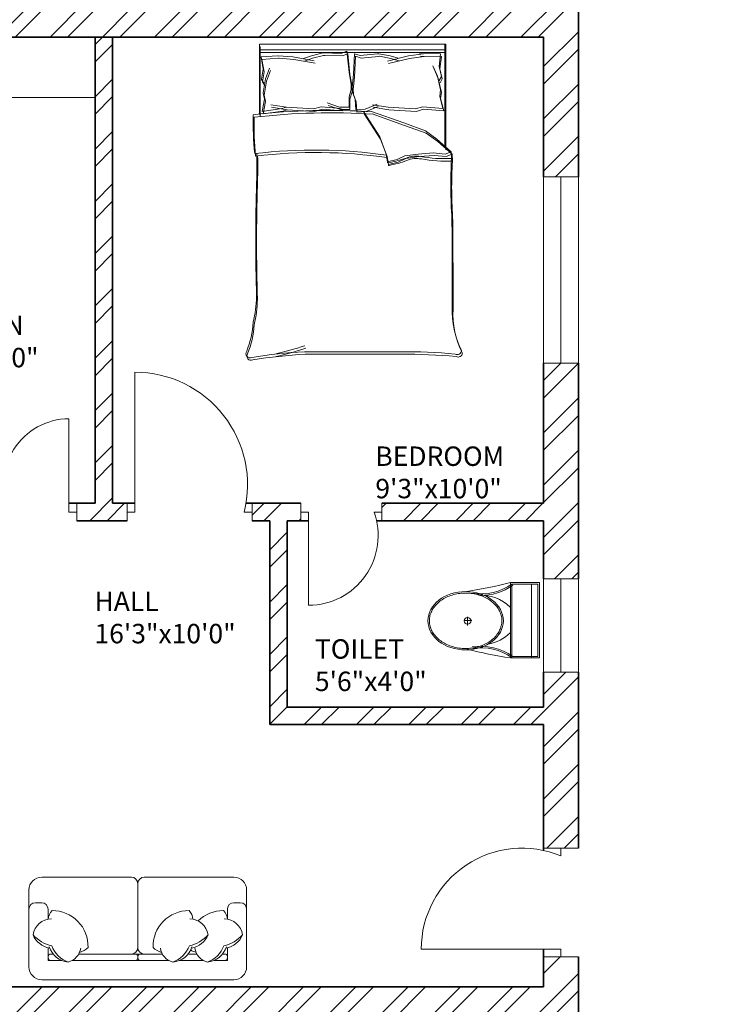
# Model space of a CAD drawing. Units: inches. Extents: x 2552 to 3217, y 1417 to 2737.
# Tile 8 of 25: x 2705 to 2885, y 1885 to 2138. Entities that reach past the tile are written whole.
import ezdxf

# ---------------------------------------------------------------- set-up
doc = ezdxf.new("R2010")
doc.units = ezdxf.units.IN
for name, color, linetype, lineweight in [('A-ANNO-DIMS', 2, 'Continuous', 18), ('A-AREA-IDEN', 7, 'Continuous', 18), ('A-DOOR', 21, 'Continuous', 18), ('A-FLOR-CASE', 9, 'Continuous', 18), ('A-FLOR-FIXT', 8, 'Continuous', 18), ('A-FURN', 8, 'Continuous', 13), ('A-GLAZ', 161, 'Continuous', 18), ('A-WALL', 7, 'Continuous', 35), ('A-WALL-PATT', 217, 'Continuous', 13)]:
    doc.layers.add(name, color=color, linetype=linetype, lineweight=lineweight)
doc.styles.get("Standard").update_dxf_attribs({"font": 'arial.ttf'})
doc.dimstyles.get("Standard").update_dxf_attribs({"dimtxt": 0.18, "dimasz": 0.18, "dimexe": 0.18, "dimexo": 0.0625, "dimgap": 0.09, "dimtad": 0, "dimtih": 1, "dimtoh": 1, "dimdec": 4, "dimzin": 0, "dimdsep": 46, "dimtxsty": 'Standard', "dimcen": 0.09, "dimadec": 0, "dimazin": 0, "dimtfac": 1, "dimtdec": 4, "dimtofl": 0, "dimtmove": 0, "dimatfit": 3, "dimfxl": 1, "dimtolj": 1, "dimtzin": 0, "dimarcsym": 0})

# ---------------------------------------------------------------- blocks, each defined once
blk = doc.blocks.new('A$C31115884')
for p, q in [((283.1, 497.7), (223.4, 497.7)), ((257.5, 466.4), (257.5, 523.2)), ((0, 200), (0, 0)), ((520, 200), (0, 200)), ((10, 190), (10, 10)), ((510, 190), (10, 190)), ((510, 10), (510, 190)), ((520, 0), (520, 200)), ((510, 54.5), (0, 54.5)), ((10, 10), (510, 10)), ((0, 0), (520, 0))]:
    blk.add_line(p, q)
blk.add_circle((255.6, 496.4), 23.6)
for centre, radius, start, end in [((2777.7, -204.6), 2807, 165.4549, 171.71327), ((3237, 905), 2807, 188.28673, 194.5451), ((-294.5, 403.3), 364.7, 324.20913, 9.34987), ((-294.5, 403.3), 374.7, 324.20913, 9.34987), ((139.5, 406.2), 293.5, 315.84364, 2.65635), ((805.8, 403.3), 374.7, 179.20365, 215.79087), ((805.8, 403.3), 364.7, 170.65013, 215.79087), ((383.6, 406.2), 293.5, 190.27735, 224.15636)]:
    blk.add_arc(centre, radius, start, end)
blk.add_ellipse((256.2, 509.9), major_axis=(0, -260.7), ratio=0.772727)
blk.add_open_spline([(256.2, 259.2), (263.1, 259.2), (270, 259.7), (287.8, 262.3), (298.7, 265.1), (319.9, 273.1), (330.2, 278.4), (350.1, 291.1), (359.7, 298.7), (377.7, 315.9), (386.2, 325.5), (401.7, 346.6), (408.8, 358.1), (421.3, 382.5), (426.8, 395.5), (435.9, 422.4), (439.5, 436.4), (444.8, 465.1), (446.5, 479.7), (447.9, 509.2), (447.6, 524), (445, 553.3), (442.7, 567.8), (436.3, 596), (432.1, 609.7), (421.9, 636), (416, 648.6), (402.5, 672.1), (395, 683), (378.6, 703), (369.8, 712.1), (351.1, 728), (341.3, 734.8), (320.9, 746.2), (310.4, 750.7), (288.9, 757.3), (278, 759.4), (256, 761), (245, 760.6), (223.1, 757.2), (212.3, 754.3), (191.1, 746.1), (180.8, 740.7), (160.9, 727.8), (151.4, 720.1), (133.5, 702.7), (125.1, 693), (109.6, 671.7), (102.6, 660.2), (90.2, 635.7), (84.9, 622.7), (76, 595.6), (72.4, 581.6), (67.2, 552.9), (65.6, 538.2), (64.4, 508.8), (64.8, 494), (67.5, 464.7), (69.9, 450.2), (76.6, 422), (80.8, 408.3), (91.1, 382.2), (97.2, 369.7), (110.8, 346.3), (118.4, 335.4), (134.8, 315.6), (143.7, 306.7), (162.4, 290.9), (172.3, 284.2), (192.8, 273), (203.3, 268.6), (224.8, 262.2), (235.8, 260.2), (249.9, 259.3), (253, 259.2), (256.2, 259.2)], degree=3, knots=[0, 0, 0, 0, 0.110105, 0.110105, 0.285049, 0.285049, 0.459994, 0.459994, 0.634938, 0.634938, 0.809882, 0.809882, 0.984827, 0.984827, 1.159771, 1.159771, 1.334715, 1.334715, 1.50966, 1.50966, 1.684604, 1.684604, 1.859549, 1.859549, 2.034493, 2.034493, 2.209437, 2.209437, 2.384382, 2.384382, 2.559326, 2.559326, 2.73427, 2.73427, 2.909215, 2.909215, 3.084159, 3.084159, 3.259103, 3.259103, 3.434048, 3.434048, 3.608992, 3.608992, 3.783936, 3.783936, 3.958881, 3.958881, 4.133825, 4.133825, 4.30877, 4.30877, 4.483714, 4.483714, 4.658658, 4.658658, 4.833603, 4.833603, 5.008547, 5.008547, 5.183491, 5.183491, 5.358436, 5.358436, 5.53338, 5.53338, 5.708324, 5.708324, 5.883269, 5.883269, 6.058213, 6.058213, 6.233158, 6.233158, 6.283185, 6.283185, 6.283185, 6.283185])
blk = doc.blocks.new('BED-DOUBLE')
for p, q in [((3.47, 63.33), (3.47, 81.44)), ((3.47, 81.44), (51.49, 81.44)), ((3.48, 63.33), (3.48, 81.44)), ((51.27, 81.44), (51.27, 54.83)), ((51.27, 81.44), (51.27, 54.83)), ((51.49, 81.44), (51.49, 80.8)), ((3.47, 79.91), (51.27, 79.91)), ((3.48, 79.91), (51.27, 79.91)), ((3.7, 62.69), (3.7, 80.8)), ((3.7, 62.69), (3.7, 80.8)), ((3.7, 79.27), (51.49, 79.27)), ((3.7, 79.27), (51.49, 79.27)), ((16.88, 78.42), (19.77, 79.14)), ((16.88, 78.42), (19.77, 79.14)), ((19.77, 79.14), (20.09, 79.14)), ((19.77, 79.14), (20.09, 79.14)), ((20.09, 79.14), (24.54, 78.99)), ((20.09, 79.14), (24.54, 78.99)), ((24.54, 78.99), (25.98, 79.57)), ((24.54, 78.99), (25.98, 79.57)), ((24.77, 78.36), (26.21, 78.93)), ((24.77, 78.36), (26.21, 78.93)), ((25.98, 79.57), (26.56, 74.22)), ((25.98, 79.57), (26.56, 74.22)), ((26.21, 78.93), (26.79, 73.58)), ((26.21, 78.93), (26.79, 73.58)), ((27.98, 78.95), (27.73, 73.58)), ((27.98, 78.95), (27.73, 73.58)), ((29.46, 78.46), (27.98, 78.95)), ((29.46, 78.46), (27.98, 78.95)), ((33.88, 78.89), (29.46, 78.46)), ((33.88, 78.89), (29.46, 78.46)), ((34.2, 78.91), (33.88, 78.89)), ((34.2, 78.91), (33.88, 78.89)), ((37.14, 78.36), (34.2, 78.91)), ((37.14, 78.36), (34.2, 78.91)), ((45.71, 78.9), (41.91, 78.37)), ((45.71, 78.9), (41.91, 78.37)), ((50.11, 78.89), (44.71, 78.98)), ((44.71, 78.98), (45.71, 78.9)), ((50.11, 78.89), (44.71, 78.98)), ((44.71, 78.98), (45.71, 78.9)), ((50.11, 78.89), (49.73, 75.68)), ((50.11, 78.89), (49.73, 75.68)), ((51.49, 80.8), (51.49, 54.19)), ((51.49, 80.8), (51.49, 54.19)), ((3.89, 78.13), (4.47, 74.95)), ((3.89, 78.13), (4.47, 74.95)), ((3.9, 78.11), (8.18, 78.43)), ((3.9, 78.11), (8.18, 78.43)), ((4.12, 77.49), (4.7, 74.31)), ((4.12, 77.49), (4.7, 74.31)), ((4.13, 77.47), (8.41, 77.8)), ((4.13, 77.47), (8.41, 77.8)), ((8.18, 78.43), (8.28, 78.42)), ((8.18, 78.43), (8.28, 78.42)), ((8.28, 78.42), (12.11, 78.13)), ((8.28, 78.42), (12.11, 78.13)), ((8.41, 77.8), (8.51, 77.78)), ((8.41, 77.8), (8.51, 77.78)), ((8.51, 77.78), (12.34, 77.49)), ((8.51, 77.78), (12.34, 77.49)), ((12.11, 78.13), (17.6, 77.12)), ((12.11, 78.13), (17.6, 77.12)), ((12.34, 77.49), (17.83, 76.48)), ((12.34, 77.49), (17.83, 76.48)), ((14.85, 77.69), (16.88, 78.42)), ((14.85, 77.69), (16.88, 78.42)), ((15.08, 77.05), (17.11, 77.78)), ((15.08, 77.05), (17.11, 77.78)), ((17.11, 77.78), (20, 78.5)), ((17.11, 77.78), (20, 78.5)), ((20, 78.5), (20.32, 78.5)), ((20, 78.5), (20.32, 78.5)), ((20.32, 78.5), (24.77, 78.36)), ((20.32, 78.5), (24.77, 78.36)), ((28.21, 78.31), (27.96, 72.94)), ((28.21, 78.31), (27.96, 72.94)), ((29.68, 77.83), (28.21, 78.31)), ((29.68, 77.83), (28.21, 78.31)), ((34.11, 78.25), (29.68, 77.83)), ((34.11, 78.25), (29.68, 77.83)), ((34.43, 78.27), (34.11, 78.25)), ((34.43, 78.27), (34.11, 78.25)), ((37.36, 77.73), (34.43, 78.27)), ((37.36, 77.73), (34.43, 78.27)), ((41.91, 78.37), (36.49, 77.02)), ((41.91, 78.37), (36.5, 77.02)), ((42.14, 77.73), (36.72, 76.38)), ((42.14, 77.73), (36.72, 76.38)), ((39.2, 77.77), (37.14, 78.36)), ((39.2, 77.77), (37.14, 78.36)), ((39.43, 77.13), (37.36, 77.73)), ((39.43, 77.13), (37.36, 77.73)), ((45.94, 78.26), (42.14, 77.73)), ((45.94, 78.26), (42.14, 77.73)), ((50.34, 78.25), (44.94, 78.34)), ((44.94, 78.34), (45.94, 78.26)), ((50.34, 78.25), (44.94, 78.34)), ((44.94, 78.34), (45.94, 78.26)), ((50.34, 78.25), (49.96, 75.04)), ((50.34, 78.25), (49.96, 75.04)), ((4.47, 74.95), (4.04, 72.34)), ((4.47, 74.95), (4.04, 72.34)), ((4.7, 74.31), (4.27, 71.7)), ((4.7, 74.31), (4.27, 71.7)), ((5.05, 72.49), (6.06, 75.24)), ((5.05, 72.49), (6.06, 75.24)), ((5.28, 71.85), (6.29, 74.6)), ((5.28, 71.85), (6.29, 74.6)), ((26.56, 74.22), (27.14, 71.04)), ((26.56, 74.22), (27.14, 71.04)), ((26.79, 73.58), (27.37, 70.4)), ((26.79, 73.58), (27.37, 70.4)), ((27.73, 73.58), (27.35, 70.37)), ((27.73, 73.58), (27.35, 70.37)), ((49.31, 73.19), (48.13, 75.86)), ((49.31, 73.19), (48.13, 75.86)), ((49.54, 72.55), (48.36, 75.23)), ((49.54, 72.55), (48.36, 75.23)), ((49.73, 75.68), (50.33, 73.1)), ((49.73, 75.68), (50.33, 73.1)), ((49.96, 75.04), (50.56, 72.47)), ((49.96, 75.04), (50.56, 72.47)), ((4.04, 72.34), (4.62, 71.33)), ((4.04, 72.34), (4.62, 71.33)), ((4.27, 71.7), (4.85, 70.69)), ((4.27, 71.7), (4.85, 70.69)), ((4.47, 68.87), (5.05, 72.49)), ((4.47, 68.87), (5.05, 72.49)), ((4.7, 68.23), (5.28, 71.85)), ((4.7, 68.23), (5.28, 71.85)), ((27.14, 71.04), (27.14, 69.74)), ((27.14, 71.04), (27.14, 69.74)), ((27.96, 72.94), (27.58, 69.73)), ((27.96, 72.94), (27.58, 69.73)), ((50.11, 69.61), (49.31, 73.19)), ((50.11, 69.61), (49.31, 73.19)), ((50.34, 68.98), (49.54, 72.55)), ((50.34, 68.98), (49.54, 72.55)), ((50.33, 73.1), (49.81, 72.06)), ((50.33, 73.1), (49.81, 72.06)), ((50.56, 72.47), (50.04, 71.42)), ((50.56, 72.47), (50.04, 71.42)), ((4.76, 67.28), (4.47, 68.87)), ((4.76, 67.28), (4.47, 68.87)), ((27.14, 69.74), (26.56, 67.86)), ((27.14, 69.74), (26.56, 67.86)), ((27.37, 69.1), (26.79, 67.22)), ((27.37, 69.1), (26.79, 67.22)), ((27.35, 70.37), (27.44, 69.07)), ((27.35, 70.37), (27.44, 69.07)), ((27.37, 70.4), (27.37, 69.1)), ((27.37, 70.4), (27.37, 69.1)), ((27.44, 69.07), (28.13, 67.23)), ((27.44, 69.07), (28.13, 67.23)), ((27.58, 69.73), (27.66, 68.43)), ((27.58, 69.73), (27.66, 68.43)), ((49.92, 68.01), (50.11, 69.61)), ((49.92, 68.01), (50.11, 69.61)), ((50.15, 67.37), (50.34, 68.98)), ((50.15, 67.37), (50.34, 68.98)), ((4.18, 64.1), (4.76, 67.28)), ((4.18, 64.1), (4.76, 67.28)), ((4.41, 63.46), (4.99, 66.64)), ((4.41, 63.46), (4.99, 66.64)), ((4.99, 66.64), (4.7, 68.23)), ((4.99, 66.64), (4.7, 68.23)), ((24.1, 65.18), (20.96, 66.27)), ((24.1, 65.18), (20.96, 66.27)), ((26.56, 67.86), (26.56, 65.18)), ((26.56, 67.86), (26.56, 65.18)), ((26.79, 67.22), (26.79, 64.54)), ((26.79, 67.22), (26.79, 64.54)), ((27.66, 68.43), (28.36, 66.59)), ((27.66, 68.43), (28.36, 66.59)), ((28.13, 67.23), (28.3, 64.55)), ((28.13, 67.23), (28.3, 64.55)), ((28.36, 66.59), (28.53, 63.91)), ((28.36, 66.59), (28.53, 63.91)), ((30.75, 64.7), (33.82, 65.99)), ((30.75, 64.7), (33.82, 65.99)), ((50.7, 64.87), (49.92, 68.01)), ((50.7, 64.87), (49.92, 68.01)), ((50.93, 64.23), (50.15, 67.37)), ((50.93, 64.23), (50.15, 67.37)), ((9.28, 64.83), (4.18, 64.1)), ((9.28, 64.83), (4.18, 64.1)), ((9.51, 64.19), (4.41, 63.46)), ((9.51, 64.19), (4.41, 63.46)), ((6.38, 65.81), (10.41, 65.15)), ((6.38, 65.81), (10.41, 65.15)), ((6.61, 65.18), (10.64, 64.51)), ((6.61, 65.18), (10.64, 64.51)), ((10.41, 65.15), (9.28, 64.83)), ((10.41, 65.15), (9.28, 64.83)), ((10.64, 64.51), (9.51, 64.19)), ((10.64, 64.51), (9.51, 64.19)), ((10.41, 65.15), (17.42, 64.72)), ((10.41, 65.15), (17.42, 64.72)), ((10.64, 64.51), (17.65, 64.08)), ((10.64, 64.51), (17.65, 64.08)), ((17.42, 64.72), (19.38, 65.27)), ((17.42, 64.72), (19.38, 65.27)), ((17.65, 64.08), (19.61, 64.63)), ((17.65, 64.08), (19.61, 64.63)), ((19.38, 65.27), (24.52, 64.87)), ((19.38, 65.27), (24.52, 64.87)), ((19.61, 64.63), (24.74, 64.23)), ((19.61, 64.63), (24.74, 64.23)), ((24.33, 64.54), (21.19, 65.63)), ((24.33, 64.54), (21.19, 65.63)), ((26.56, 65.18), (24.1, 65.18)), ((26.56, 65.18), (24.1, 65.18)), ((26.79, 64.54), (24.33, 64.54)), ((26.79, 64.54), (24.33, 64.54)), ((28.3, 64.55), (30.75, 64.7)), ((28.3, 64.55), (30.75, 64.7)), ((28.53, 63.91), (30.98, 64.06)), ((28.53, 63.91), (30.98, 64.06)), ((30.26, 64.06), (34.45, 57.57)), ((30.26, 64.06), (34.45, 57.57)), ((30.49, 63.42), (34.68, 56.93)), ((30.49, 63.42), (34.68, 56.93)), ((30.98, 64.06), (34.05, 65.35)), ((30.98, 64.06), (34.05, 65.35)), ((40.64, 61.13), (32.31, 64.06)), ((40.64, 61.13), (32.31, 64.06)), ((40.87, 60.49), (32.53, 63.42)), ((40.87, 60.49), (32.53, 63.42)), ((32.56, 65.81), (36.6, 65.15)), ((32.56, 65.81), (36.6, 65.15)), ((32.79, 65.18), (36.82, 64.51)), ((32.79, 65.18), (36.82, 64.51)), ((36.6, 65.15), (43.61, 64.72)), ((36.6, 65.15), (43.61, 64.72)), ((36.82, 64.51), (43.83, 64.08)), ((36.82, 64.51), (43.83, 64.08)), ((43.61, 64.72), (45.57, 65.27)), ((43.61, 64.72), (45.57, 65.27)), ((43.83, 64.08), (45.79, 64.63)), ((43.83, 64.08), (45.79, 64.63)), ((45.57, 65.27), (50.7, 64.87)), ((45.57, 65.27), (50.7, 64.87)), ((45.79, 64.63), (50.93, 64.23)), ((45.79, 64.63), (50.93, 64.23)), ((46.22, 59.11), (40.64, 61.13)), ((46.22, 59.11), (40.64, 61.13)), ((46.45, 58.48), (40.87, 60.49)), ((46.45, 58.48), (40.87, 60.49)), ((49.16, 56.95), (46.22, 59.11)), ((49.16, 56.95), (46.22, 59.11)), ((49.39, 56.31), (46.45, 58.48)), ((49.39, 56.31), (46.45, 58.48)), ((34.45, 57.57), (36.15, 53.08)), ((34.45, 57.57), (36.15, 53.08)), ((34.68, 56.93), (36.38, 52.44)), ((34.68, 56.93), (36.38, 52.44)), ((52.87, 53.7), (49.16, 56.95)), ((52.87, 53.7), (49.16, 56.95)), ((53.1, 53.06), (49.39, 56.31)), ((53.1, 53.06), (49.39, 56.31)), ((44.36, 53.08), (48.23, 53.39)), ((44.36, 53.08), (48.23, 53.39)), ((48.23, 53.39), (51.33, 53.08)), ((48.23, 53.39), (51.33, 53.08)), ((51.33, 53.08), (52.87, 53.7)), ((51.33, 53.08), (52.87, 53.7)), ((52.95, 51.95), (52.87, 53.7, 3.87)), ((52.95, 51.95), (52.87, 53.7, 3.87)), ((36.15, 53.08), (36.46, 51.07)), ((36.15, 53.08), (36.46, 51.07)), ((36.38, 52.44), (36.69, 50.43)), ((36.38, 52.44), (36.69, 50.43)), ((36.46, 51.07), (38.94, 51.69)), ((36.46, 51.07), (38.94, 51.69)), ((36.69, 50.43), (39.17, 51.05)), ((36.69, 50.43), (39.17, 51.05)), ((38.94, 51.69), (40.95, 52.61)), ((38.94, 51.69), (40.95, 52.61)), ((39.17, 51.05), (41.18, 51.97)), ((39.17, 51.05), (41.18, 51.97)), ((40.95, 52.61), (44.36, 53.08)), ((40.95, 52.61), (44.36, 53.08)), ((41.18, 51.97), (44.59, 52.44)), ((41.18, 51.97), (44.59, 52.44)), ((44.59, 52.44), (48.46, 52.75)), ((44.59, 52.44), (48.46, 52.75)), ((48.46, 52.75), (51.56, 52.44)), ((48.46, 52.75), (51.56, 52.44)), ((51.56, 52.44), (53.1, 53.06)), ((51.56, 52.44), (53.1, 53.06)), ((53.18, 51.31), (53.1, 53.06, 3.87)), ((53.18, 51.31), (53.1, 53.06, 3.87)), ((15.06, 2.2), (39.68, 2.2)), ((15.06, 2.2), (39.68, 2.2)), ((15.29, 1.56), (39.91, 1.56)), ((15.29, 1.56), (39.91, 1.56))]:
    blk.add_line(p, q)
for centre, radius, start, end in [((21.36, -100.61), 164.97, 86.0865, 96.7821), ((21.36, -100.61), 164.97, 86.0865, 96.7821), ((21.59, -101.25), 164.97, 86.0865, 96.7821), ((21.59, -101.25), 164.97, 86.0865, 96.7821), ((85.16, 61.35), 83.31, 178.7218, 185.604), ((85.16, 61.35), 83.31, 178.7218, 185.604), ((85.39, 60.71), 83.31, 178.7218, 185.604), ((85.39, 60.71), 83.31, 178.7218, 185.604), ((17.76, -74.87), 129.02, 81.7845, 96.9006), ((17.76, -74.87), 129.02, 81.7845, 96.9006), ((17.98, -75.51), 129.02, 81.7845, 96.9006), ((17.98, -75.51), 129.02, 81.7845, 96.9006), ((-167.31, 50.27), 170.11, 358.4762, 1.0082), ((-167.31, 50.27), 170.11, 358.4762, 1.0082), ((-167.08, 49.63), 170.11, 358.4762, 1.0082), ((-167.08, 49.63), 170.11, 358.4762, 1.0082), ((36.64, 51), 0.185, 160.2464, 271.1377), ((36.64, 51), 0.185, 160.2464, 271.1377), ((31.15, 79.96), 29.65, 280.6617, 289.8806), ((31.15, 79.96), 29.65, 280.6617, 289.8806), ((31.38, 79.32), 29.65, 280.6617, 289.8806), ((31.38, 79.32), 29.65, 280.6617, 289.8806), ((43.74, 46.38), 6.22, 78.6608, 113.7384), ((43.74, 46.38), 6.22, 78.6608, 113.7384), ((43.97, 45.74), 6.22, 78.6608, 113.7384), ((43.97, 45.74), 6.22, 78.6608, 113.7384), ((51.33, 88.1), 36.18, 259.8763, 272.5657), ((51.33, 88.1), 36.18, 259.8763, 272.5657), ((51.56, 87.46), 36.18, 259.8763, 272.5657), ((51.56, 87.46), 36.18, 259.8763, 272.5657), ((182.27, 45.13), 129.5, 176.9791, 183.8365), ((182.27, 45.13), 129.5, 176.9791, 183.8365), ((182.49, 44.49), 129.5, 176.9791, 183.8365), ((182.49, 44.49), 129.5, 176.9791, 183.8365), ((36.86, 50.36), 0.185, 160.2464, 271.1377), ((36.86, 50.36), 0.185, 160.2464, 271.1377), ((484.82, 30.83), 482.31, 178.2277, 181.7185), ((484.82, 30.83), 482.31, 178.2277, 181.7185), ((485.05, 30.19), 482.31, 178.2277, 181.7185), ((485.05, 30.19), 482.31, 178.2277, 181.7185), ((-4508.74, 13.62), 4561.86, 0.00217, 0.28689), ((-4508.74, 13.62), 4561.86, 0.00217, 0.28689), ((-4508.51, 12.98), 4561.86, 0.00217, 0.28689), ((-4508.52, 12.98), 4561.86, 0.00217, 0.28689), ((-26.9, 16.93), 29.63, 346.0648, 358.9113), ((-26.9, 16.93), 29.63, 346.0648, 358.9113), ((-26.67, 16.29), 29.63, 346.0648, 358.9113), ((-26.67, 16.29), 29.63, 346.0648, 358.9113), ((76.16, 12.78), 23.07, 177.4714, 206.4681), ((76.16, 12.78), 23.07, 177.4714, 206.4681), ((76.39, 12.14), 23.07, 177.4714, 206.4681), ((76.39, 12.14), 23.07, 177.4714, 206.4681), ((-21.66, 11.17), 23.56, 337.9751, 356.652), ((-21.66, 11.17), 23.56, 337.9751, 356.652), ((-21.43, 10.53), 23.56, 337.9751, 356.652), ((-21.43, 10.53), 23.56, 337.9751, 356.652), ((-17.22, 105.16), 106.46, 283.3832, 287.7053), ((-17.22, 105.16), 106.46, 283.3832, 287.7053), ((-16.99, 104.52), 106.46, 283.3832, 287.7053), ((-16.99, 104.52), 106.46, 283.3832, 287.7053), ((1.09, 1.73), 1.09, 146.1736, 293.4781), ((1.09, 1.73), 1.09, 146.1736, 293.4781), ((1.32, 1.09), 1.09, 146.1736, 293.4781), ((1.32, 1.09), 1.09, 146.1736, 293.4781), ((21.43, -119.39), 121.76, 92.9958, 99.4091), ((21.43, -119.39), 121.76, 92.9958, 99.4091), ((21.66, -120.03), 121.76, 92.9958, 99.4091), ((21.65, -120.03), 121.76, 92.9958, 99.4091), ((41.15, -130.83), 133.04, 84.4998, 90.6351), ((41.15, -130.83), 133.04, 84.4998, 90.6351), ((41.38, -131.47), 133.04, 84.4998, 90.6351), ((41.38, -131.47), 133.04, 84.4998, 90.6351), ((54.41, 2.57), 1.1, 242.6588, 356.02), ((54.41, 2.57), 1.1, 242.6588, 356.02), ((54.64, 1.93), 1.1, 242.6588, 356.02), ((54.64, 1.93), 1.1, 242.6588, 356.02)]:
    blk.add_arc(centre, radius, start, end)
blk = doc.blocks.new('WIN-48')
for p, q in [((4.5, 48), (0, 48)), ((0, 48), (9, 48)), ((0, 48), (0, 0)), ((4.5, 0), (4.5, 48)), ((9, 48), (9, 0)), ((0, 0), (9, 0)), ((9, 0), (4.5, 0))]:
    blk.add_line(p, q)
blk = doc.blocks.new('WIN-24')
for p, q in [((0, 24), (9, 24)), ((0, 24), (0, 0)), ((9, 24), (4.5, 24)), ((4.5, 24), (4.5, 0)), ((9, 24), (9, 0)), ((4.5, 0), (0, 0)), ((0, 0), (9, 0))]:
    blk.add_line(p, q)
blk = doc.blocks.new('*D64')
at = {"layer": 'A-ANNO-DIMS', "color": 0, "lineweight": -2, "transparency": 16777216}
for p, q in [((2646.35, 1551.58), (2646.35, 2709.49)), ((2646.53, 2709.31), (2802.77, 2709.31)), ((2959.93, 2709.31), (2803.69, 2709.31)), ((2960.11, 1551.58), (2960.11, 2709.49))]:
    blk.add_line(p, q, dxfattribs=at)
at = {"layer": 'A-ANNO-DIMS', "color": 0, "transparency": 16777216}
for points in [[(2646.53, 2709.34), (2646.53, 2709.28), (2646.35, 2709.31)], [(2959.93, 2709.34), (2959.93, 2709.28), (2960.11, 2709.31)]]:
    blk.add_solid(points, dxfattribs=at)
at = {"layer": 'Defpoints', "color": 0, "transparency": 16777216}
for p in [(2960.11, 2709.31), (2646.35, 1551.51), (2960.11, 1551.51)]:
    blk.add_point(p, dxfattribs=at)
at = {"layer": 'A-ANNO-DIMS', "color": 0, "transparency": 16777216, "insert": (2803.23, 2709.31), "char_height": 0.18, "attachment_point": 5}
blk.add_mtext('\\A1;313.76', dxfattribs=at)

msp = doc.modelspace()

# ---------------------------------------------------------------- hatches: boundary and pattern name
at = {"layer": 'A-WALL-PATT'}
h = msp.add_hatch(dxfattribs=at)
h.set_pattern_fill('ANSI32', color=256)
h.paths.add_polyline_path([(2756.676, 2649.5125), (2637.3535, 2649.5125), (2637.3535, 2617.9626), (2641.8535, 2617.9626), (2646.3535, 2617.9626), (2646.3535, 2640.5125), (2724.3535, 2640.5125), (2724.3535, 2520.5125), (2720.299, 2520.5125), (2720.299, 2516.0125), (2733.4075, 2516.0125), (2733.4075, 2518.2213), (2733.4075, 2520.5125), (2728.8535, 2520.5125), (2728.8535, 2640.5125), (2756.676, 2640.5125)])
h.paths.add_polyline_path([(2848.8535, 2649.5125), (2804.676, 2649.5125), (2804.676, 2640.5125), (2839.8535, 2640.5125), (2839.8535, 2598.3517), (2848.8535, 2598.3517)])
h.paths.add_polyline_path([(2646.3535, 2516.0125), (2697.9593, 2516.0125), (2697.9593, 2518.2625), (2697.9593, 2520.5125), (2646.3535, 2520.5125), (2646.3535, 2581.9626), (2637.3535, 2581.9626), (2637.3535, 2364.3298), (2646.3535, 2364.3298), (2646.3535, 2387.0125), (2724.3535, 2387.0125), (2724.3535, 2267.0125), (2721.0443, 2267.0125), (2721.0443, 2262.5125), (2733.7854, 2262.5125), (2733.7854, 2264.7625), (2733.7854, 2267.0125), (2728.8535, 2267.0125), (2728.8535, 2387.0125), (2839.8535, 2387.0125), (2839.8535, 2363.8387), (2848.8535, 2363.8387), (2848.8535, 2403.7415), (2844.3535, 2403.7415), (2839.8535, 2403.7415), (2839.8535, 2396.0125), (2646.3535, 2396.0125)])
h.paths.add_polyline_path([(2848.8535, 2550.3517), (2844.3535, 2550.3517), (2839.8535, 2550.3517), (2839.8535, 2520.5125), (2801.9195, 2520.5125), (2801.9195, 2518.2625), (2801.9195, 2516.0125), (2839.8535, 2516.0125), (2839.8535, 2507.5813), (2848.8535, 2507.5813)], flags=17)
h.paths.add_polyline_path([(2848.8535, 2483.5813), (2844.3535, 2483.5813), (2839.8535, 2483.5813), (2839.8535, 2468.0125), (2773.8535, 2468.0125), (2773.8535, 2516.0125), (2778.1336, 2516.0125), (2778.1336, 2520.5125), (2766.696, 2520.5125), (2766.696, 2518.2625), (2766.696, 2516.0125), (2769.3535, 2516.0125), (2769.3535, 2463.5125), (2839.8535, 2463.5125), (2839.8535, 2431.0782), (2848.8535, 2431.0782)], flags=17)
h.paths.add_polyline_path([(2917.8535, 2569.2764), (2913.3535, 2569.2764), (2908.8535, 2569.2764), (2908.8535, 2433.001), (2917.8535, 2433.001), (2917.8535, 2516.0125), (2967.486, 2516.0125), (2967.486, 2520.5125), (2917.8535, 2520.5125)])
h.paths.add_polyline_path([(3000.3535, 2640.5125), (2995.8535, 2640.5125), (2995.8535, 2520.5125), (2990.688, 2520.5125), (2990.688, 2516.0125), (3004.0844, 2516.0125), (3004.0844, 2518.2625), (3004.0844, 2520.5125), (3000.3535, 2520.5125)])
h.paths.add_polyline_path([(3120.3535, 2561.3689), (3115.8535, 2561.3689), (3111.3535, 2561.3689), (3111.3535, 2520.5125), (3070.9814, 2520.5125), (3070.9814, 2518.2625), (3070.9814, 2516.0125), (3111.3535, 2516.0125), (3111.3535, 2505.1841), (3120.3535, 2505.1841)])
h.paths.add_polyline_path([(3120.3535, 2481.1841), (3115.8535, 2481.1841), (3111.3535, 2481.1841), (3111.3535, 2468.0125), (3045.3535, 2468.0125), (3045.3535, 2516.0125), (3048.9787, 2516.0125), (3048.9787, 2520.5125), (3036.3395, 2520.5125), (3036.3395, 2516.0125), (3040.8535, 2516.0125), (3040.8535, 2463.5125), (3111.3535, 2463.5125), (3111.3535, 2396.0125), (2917.8535, 2396.0125), (2917.8535, 2403.4124), (2913.3535, 2403.4124), (2908.8535, 2403.4124), (2908.8535, 2182.5756), (2917.8535, 2182.5756), (2917.8535, 2262.5125), (2968.001, 2262.5125), (2968.001, 2264.7625), (2968.001, 2267.0125), (2917.8535, 2267.0125), (2917.8535, 2387.0125), (3111.3535, 2387.0125), (3111.3535, 2352.2435), (3120.3535, 2352.2435)])
h.paths.add_polyline_path([(3120.3535, 2304.2435), (3115.8535, 2304.2435), (3111.3535, 2304.2435), (3111.3535, 2267.0125), (3073.8616, 2267.0125), (3073.8616, 2264.7625), (3073.8616, 2262.5125), (3111.3535, 2262.5125), (3111.3535, 2252.376), (3120.3535, 2252.376)], flags=17)
h.paths.add_polyline_path([(3120.3535, 2228.376), (3115.8535, 2228.376), (3111.3535, 2228.376), (3111.3535, 2214.5125), (3045.3535, 2214.5125), (3045.3535, 2262.5125), (3049.3096, 2262.5125), (3049.3096, 2267.0125), (3035.0125, 2267.0125), (3035.0125, 2262.5125), (3040.8535, 2262.5125), (3040.8535, 2210.0125), (3111.3535, 2210.0125), (3111.3535, 2142.5125), (2917.8535, 2142.5125), (2917.8535, 2150.2408), (2913.3535, 2150.2408), (2908.8535, 2150.2408), (2908.8535, 1924.9905), (2917.8535, 1924.9905), (2917.8535, 2009.0125), (2971.959, 2009.0125), (2971.959, 2011.2625), (2971.959, 2013.5125), (2917.8535, 2013.5125), (2917.8535, 2133.5125), (2995.8535, 2133.5125), (2995.8535, 2013.5125), (2992.1797, 2013.5125), (2992.1797, 2009.0125), (3004.3344, 2009.0125), (3004.3344, 2011.2625), (3004.3344, 2013.5125), (3000.3535, 2013.5125), (3000.3535, 2133.5125), (3111.3535, 2133.5125), (3111.3535, 2115.0291), (3120.3535, 2115.0291)])
h.paths.add_polyline_path([(3000.3535, 2387.0125), (2995.8535, 2387.0125), (2995.8535, 2267.0125), (2991.3326, 2267.0125), (2991.3326, 2262.5125), (3004.1044, 2262.5125), (3004.1044, 2264.7625), (3004.1044, 2267.0125), (3000.3535, 2267.0125)], flags=17)
h.paths.add_polyline_path([(3120.3535, 1973.2388), (3115.8535, 1973.2388), (3111.3535, 1973.2388), (3111.3535, 1961.0125), (3045.3535, 1961.0125), (3045.3535, 2009.0125), (3048.9101, 2009.0125), (3048.9101, 2013.5125), (3037.105, 2013.5125), (3037.105, 2011.2625), (3037.105, 2009.0125), (3040.8535, 2009.0125), (3040.8535, 1956.5125), (3111.3535, 1956.5125), (3111.3535, 1889.0125), (2917.8535, 1889.0125), (2917.8535, 1895.7215), (2913.3535, 1895.7215), (2908.8535, 1895.7215), (2908.8535, 1844.2217), (2917.8535, 1844.2217), (2917.8535, 1880.0125), (3111.3535, 1880.0125), (3111.3535, 1846.9541), (3120.3535, 1846.9541)])
h.paths.add_polyline_path([(3120.3535, 2067.0291), (3111.3535, 2067.0291), (3111.3535, 2013.5125), (3071.3001, 2013.5125), (3071.3001, 2009.0125), (3111.3535, 2009.0125), (3111.3535, 1997.2388), (3120.3535, 1997.2388)], flags=0)
h.paths.add_polyline_path([(3120.3535, 1798.9541), (3115.8535, 1798.9541), (3111.3535, 1798.9541), (3111.3535, 1760.0125), (3071.2497, 1760.0125), (3071.2497, 1757.7625), (3071.2497, 1755.5125), (3111.3535, 1755.5125), (3111.3535, 1746.162), (3120.3535, 1746.2478)])
h.paths.add_polyline_path([(3120.3535, 1722.2049), (3111.3535, 1722.2049), (3111.3535, 1707.5125), (3045.3535, 1707.5125), (3045.3535, 1755.5125), (3048.6624, 1755.5125), (3048.6624, 1760.0125), (3035.3703, 1760.0125), (3035.3703, 1755.5125), (3040.8535, 1755.5125), (3040.8535, 1703.0125), (3111.3535, 1703.0125), (3111.3535, 1635.5125), (2917.8535, 1635.5125), (2917.8535, 1643.1366), (2913.3535, 1643.1366), (2908.8535, 1643.1366), (2908.8535, 1626.5125), (3120.3535, 1626.5125)])
h.paths.add_polyline_path([(2917.8535, 1755.5125), (2973.2287, 1755.5125), (2973.2287, 1757.7625), (2973.2287, 1760.0125), (2917.8535, 1760.0125), (2917.8535, 1808.2217), (2913.3535, 1808.2217), (2908.8535, 1808.2217), (2908.8535, 1676.1665), (2917.8535, 1676.1665)])
h.paths.add_polyline_path([(3000.3535, 1880.0125), (2995.8535, 1880.0125), (2995.8535, 1760.0125), (2992.9329, 1760.0125), (2992.9329, 1755.5125), (3003.8766, 1755.5125), (3003.8766, 1757.7625), (3003.8766, 1760.0125), (3000.3535, 1760.0125)])
h.paths.add_polyline_path([(2848.8535, 1896.6971), (2844.3535, 1896.6971), (2839.8535, 1896.6971), (2839.8535, 1889.0125), (2646.3535, 1889.0125), (2646.3535, 2009.0125), (2700.5253, 2009.0125), (2700.5253, 2011.2625), (2700.5253, 2013.5125), (2646.3535, 2013.5125), (2646.3535, 2053.1812), (2641.8535, 2053.1812), (2637.3535, 2053.1812), (2637.3535, 1836.254), (2646.3535, 1836.254), (2646.3535, 1880.0125), (2724.3535, 1880.0125), (2724.3535, 1760.0125), (2721.2473, 1760.0125), (2721.2473, 1755.5125), (2731.9187, 1755.5125), (2731.9187, 1757.7625), (2731.9187, 1760.0125), (2728.8535, 1760.0125), (2728.8535, 1880.0125), (2839.8535, 1880.0125), (2839.8535, 1840.3813), (2848.8535, 1840.3813)])
h.paths.add_polyline_path([(2848.8535, 1792.3813), (2844.3535, 1792.3813), (2839.8535, 1792.3813), (2839.8535, 1760.0125), (2797.8845, 1760.0125), (2797.8845, 1755.5125), (2839.8535, 1755.5125), (2839.8535, 1743.3688), (2844.3535, 1743.3688), (2848.8535, 1743.3688)], flags=0)
h.paths.add_polyline_path([(2848.8535, 1719.3688), (2844.3535, 1719.3688), (2839.8535, 1719.3688), (2839.8535, 1707.5125), (2773.8535, 1707.5125), (2773.8535, 1755.5125), (2777.716, 1755.5125), (2777.716, 1760.0125), (2760.9247, 1760.0125), (2760.9247, 1757.9721), (2760.9247, 1755.5125), (2769.3535, 1755.5125), (2769.3535, 1703.0125), (2839.8535, 1703.0125), (2839.8535, 1673.0277), (2848.8535, 1672.9407)], flags=0)
h.paths.add_polyline_path([(2646.3535, 1755.5125), (2702.9171, 1755.5125), (2702.9171, 1757.7625), (2702.9171, 1760.0125), (2646.3535, 1760.0125), (2646.3535, 1800.254), (2641.8535, 1800.254), (2637.3535, 1800.254), (2637.3535, 1626.5125), (2848.8535, 1626.5125), (2848.8535, 1643.1187), (2844.3535, 1643.1187), (2839.8535, 1643.1187), (2839.8535, 1635.5125), (2646.3535, 1635.5125)])
h.paths.add_polyline_path([(2848.8535, 2148.8427), (2844.3535, 2148.8427), (2839.8535, 2148.8427), (2839.8535, 2142.5125), (2646.3535, 2142.5125), (2646.3535, 2262.5125), (2701.3562, 2262.5125), (2701.3562, 2264.7625), (2701.3562, 2267.0125), (2646.3535, 2267.0125), (2646.3535, 2328.3298), (2637.3535, 2328.3298), (2637.3535, 2089.1812), (2646.3535, 2089.1812), (2646.3535, 2133.5125), (2839.8535, 2133.5125), (2839.8535, 2097.5966), (2848.8535, 2097.5966)])
h.paths.add_polyline_path([(2728.8535, 2133.5125), (2724.3535, 2133.5125), (2724.3535, 2013.5125), (2719.6039, 2013.5125), (2719.6039, 2009.0125), (2732.5784, 2009.0125), (2732.5784, 2011.2625), (2732.5784, 2013.5125), (2728.8535, 2013.5125)])
h.paths.add_polyline_path([(2848.8535, 1970.0557), (2844.3535, 1970.0557), (2839.8535, 1970.0557), (2839.8535, 1961.0125), (2773.8535, 1961.0125), (2773.8535, 2009.0125), (2777.3388, 2009.0125), (2777.3388, 2013.5125), (2764.7681, 2013.5125), (2764.7681, 2009.0125), (2769.3535, 2009.0125), (2769.3535, 1956.5125), (2839.8535, 1956.5125), (2839.8535, 1924.7199), (2848.8535, 1924.7199)], flags=17)
h.paths.add_polyline_path([(2848.8535, 2049.5966), (2844.3535, 2049.5966), (2839.8535, 2049.5966), (2839.8535, 2013.5125), (2798.198, 2013.5125), (2798.198, 2011.2625), (2798.198, 2009.0125), (2839.8535, 2009.0125), (2839.8535, 1994.0557), (2848.8535, 1994.0557)], flags=17)
h.paths.add_polyline_path([(2848.8535, 2315.8387), (2839.8535, 2315.8387), (2839.8535, 2267.0125), (2799.3375, 2267.0125), (2799.3375, 2264.7625), (2799.3375, 2262.5125), (2839.8535, 2262.5125), (2839.8535, 2253.2843), (2848.8535, 2253.2843)], flags=17)
h.paths.add_polyline_path([(2848.8535, 2229.2843), (2839.8535, 2229.2843), (2839.8535, 2177.6936), (2848.8535, 2177.6936)], flags=17)
h.paths.add_polyline_path([(2839.8535, 2214.5125), (2773.8535, 2214.5125), (2773.8535, 2262.5125), (2777.6984, 2262.5125), (2777.6984, 2267.0125), (2763.8226, 2267.0125), (2763.8226, 2262.5125), (2769.3535, 2262.5125), (2769.3535, 2210.0125), (2839.8535, 2210.0125)], flags=17)
h.paths.add_polyline_path([(3050.32, 2520.2817), (3088.9114, 2520.2817), (3088.9114, 2538.939), (3050.32, 2538.939)], flags=9)

# ---------------------------------------------------------------- linework, layer by layer
at = {"layer": 'A-DOOR'}
for p, q in [((2734.5784, 2011.2625), (2734.5784, 2047.2625)), ((2717.6039, 2011.2625), (2717.6039, 2035.2625)), ((2719.6039, 2013.5125), (2719.6039, 2009.0125)), ((2732.5784, 2013.5125), (2732.5784, 2009.0125)), ((2764.7681, 2013.5125), (2764.7681, 2009.0125)), ((2777.3388, 2009.0125), (2777.3388, 2013.5125)), ((2777.3388, 2013.5125), (2777.3388, 2011.2625)), ((2798.198, 2009.0125), (2798.198, 2013.5125)), ((2798.198, 2013.5125), (2798.198, 2011.2625)), ((2719.6039, 2011.2625), (2717.6039, 2011.2625)), ((2719.6039, 2009.0125), (2719.6039, 2011.2625)), ((2732.5784, 2009.0125), (2732.5784, 2011.2625)), ((2732.5784, 2011.2625), (2734.5784, 2011.2625)), ((2764.7681, 2011.2625), (2762.7681, 2011.2625)), ((2764.7681, 2009.0125), (2764.7681, 2011.2625)), ((2777.3388, 2011.2625), (2779.3388, 2011.2625)), ((2779.3388, 2011.2625), (2779.3388, 1987.2625)), ((2798.198, 2011.2625), (2796.198, 2011.2625)), ((2839.8535, 1926.6737), (2839.8535, 1926.6737)), ((2839.8535, 1924.7199), (2848.8535, 1924.7199)), ((2848.8535, 1924.7199), (2844.3535, 1924.7199)), ((2844.3535, 1924.7199), (2844.3535, 1922.7199)), ((2848.8535, 1924.7199), (2848.8535, 1924.7199)), ((2844.3535, 1898.6971), (2808.3535, 1898.6971)), ((2839.8535, 1896.6971), (2848.8535, 1896.6971)), ((2844.3535, 1896.6971), (2844.3535, 1898.6971)), ((2848.8535, 1896.6971), (2844.3535, 1896.6971))]:
    msp.add_line(p, q, dxfattribs=at)
for centre, radius, start, end in [((2734.5784, 2018.2255), 29.037, 346.125389, 90), ((2717.6039, 2018.5258), 16.7367, 90, 205.719887), ((2779.3388, 2005.184), 17.9215, 270, 19.826547), ((2834.3688, 1898.6971), 26.0153, 67.430562, 180)]:
    msp.add_arc(centre, radius, start, end, dxfattribs=at)
at = {"layer": 'A-FLOR-CASE'}
msp.add_line((2663.7921, 2118.0143), (2724.3535, 2118.0143), dxfattribs=at)
at = {"layer": 'A-FURN', "ltscale": 0.03}
msp.add_lwpolyline([(2733.6932, 1917.2476, -0.41421356), (2735.3428, 1915.5981, -0.41421356), (2736.9924, 1917.2476), (2760.0863, 1917.2476, -0.41421356), (2763.3854, 1913.9485), (2763.3854, 1894.1537, -0.41421356), (2760.0863, 1890.8546), (2710.5994, 1890.8546, -0.41421356), (2707.3002, 1894.1537), (2707.3002, 1913.9485, -0.41421356), (2710.5994, 1917.2476), (2733.6932, 1917.2476, -0.41421356), (2735.3428, 1915.5981, -0.41421356), (2736.9924, 1917.2476)], format="xyb", dxfattribs=at)
at = {"layer": 'A-FURN'}
for points in [[(2733.6932, 1897.4529, 0.41421356), (2735.3428, 1899.1024), (2735.3428, 1915.5981, 0.41421356)], [(2736.9924, 1897.4529, -0.41421356), (2735.3428, 1899.1024), (2735.3428, 1915.5981, -0.41421356)], [(2707.3002, 1908.9998, -0.41421356), (2708.9498, 1910.6494), (2710.5994, 1910.6494, -0.41421356), (2712.2489, 1908.9998), (2712.2489, 1906.444)], [(2758.4367, 1906.444), (2758.4367, 1908.9998, -0.41421356), (2760.0863, 1910.6494), (2761.7358, 1910.6494, -0.41421356), (2763.3854, 1908.9998)], [(2713.0767, 1906.5439, 0.35677236), (2708.3501, 1902.386, 0.24954205), (2712.6329, 1898.9595, -9.61688035)], [(2712.2453, 1906.4433, -0.16554063), (2713.2658, 1908.6228, -0.42598917), (2722.5301, 1899.173, -0.12152332), (2720.3309, 1897.8705, 7.11546429)], [(2749.5542, 1906.4433, 0.16554063), (2748.5337, 1908.6228, 0.42598917), (2739.2694, 1899.173, 0.12152332), (2741.4686, 1897.8705, -7.11546429)], [(2748.7227, 1906.5439, -0.35677236), (2753.4494, 1902.386, -0.24954205), (2749.1666, 1898.9595, 9.61688035)], [(2758.4403, 1906.4433, 0.16554063), (2757.4198, 1908.6228, 0.20023115), (2750.8717, 1905.9684, 0.12152332)], [(2757.6089, 1906.5439, -0.35677236), (2762.3356, 1902.386, -0.24954205), (2758.0528, 1898.9595, 9.61688035)], [(2708.3501, 1902.386, 0.14772988), (2713.1713, 1899.551, 0.21334276), (2717.4253, 1895.3931, 0.17866181)], [(2753.4494, 1902.386, -0.14772988), (2748.6282, 1899.551, -0.21334276), (2744.3742, 1895.3931, -0.17866181)], [(2762.3356, 1902.386, -0.14772988), (2757.5144, 1899.551, -0.21334276), (2753.2604, 1895.3931, -0.17866181)], [(2712.5052, 1899.3251, 0.30666349), (2717.4253, 1895.3931, 0.30632997), (2720.6394, 1898.984, -0.87284716)], [(2733.6932, 1897.4529, 0.41421356), (2735.3428, 1899.1024)], [(2736.9924, 1897.4529, -0.41421356), (2735.3428, 1899.1024)], [(2749.2943, 1899.3251, -0.30666349), (2744.3742, 1895.3931, -0.30632997), (2741.1601, 1898.984, 0.87284716)], [(2758.1804, 1899.3251, -0.30666349), (2753.2604, 1895.3931, -0.30632997), (2750.0462, 1898.984, 0.87284716)], [(2754.9665, 1895.8033), (2758.4367, 1895.8033), (2758.4367, 1899.0451, -0.41421356)], [(2713.5077, 1897.4529), (2712.9087, 1897.4529, 0.41421356), (2712.2489, 1896.793), (2712.2489, 1896.4631, 0.41421356), (2712.9087, 1895.8033)], [(2718.4634, 1895.8033), (2734.683, 1895.8033, 0.41421356), (2735.3428, 1896.4631), (2735.3428, 1896.793, 0.41421356), (2734.683, 1897.4529), (2720.1244, 1897.4529, 0.41421356)], [(2743.3361, 1895.8033), (2736.0026, 1895.8033, -0.41421356), (2735.3428, 1896.4631), (2735.3428, 1896.793, -0.41421356), (2736.0026, 1897.4529), (2741.6751, 1897.4529, -0.41421356)], [(2748.2918, 1897.4529), (2750.5612, 1897.4529, -0.41421356)], [(2748.9717, 1898.5154, 0.07186538), (2750.3547, 1897.8705, -7.11546429)], [(2757.1779, 1897.4529), (2757.7769, 1897.4529, -0.41421356), (2758.4367, 1896.793), (2758.4367, 1896.4631, -0.41421356), (2757.7769, 1895.8033)], [(2712.9087, 1895.8033), (2715.7191, 1895.8033, 0.41421356)], [(2752.2222, 1895.8033), (2746.0803, 1895.8033, -0.41421356)], [(2757.7769, 1895.8033), (2754.9665, 1895.8033, -0.41421356)]]:
    msp.add_lwpolyline(points, format="xyb", dxfattribs=at)
for points in [[(2712.2489, 1899.0451), (2712.2489, 1895.8033), (2715.7191, 1895.8033)], [(2718.4634, 1895.8033), (2743.3361, 1895.8033)], [(2746.0803, 1895.8033), (2752.2222, 1895.8033)]]:
    msp.add_lwpolyline(points, dxfattribs=at)
msp.add_lwpolyline([(2734.683, 1895.8033), (2736.0026, 1895.8033, -0.41421356), (2735.3428, 1896.4631), (2735.3428, 1896.793, -0.41421356), (2736.0026, 1897.4529), (2734.683, 1897.4529, -0.41421356), (2735.3428, 1896.793), (2735.3428, 1896.4631, -0.41421356)], format="xyb", close=True, dxfattribs=at)
at = {"layer": 'A-GLAZ'}
msp.add_line((2839.8535, 2049.5966), (2839.8535, 2049.5966), dxfattribs=at)
at = {"layer": 'A-WALL'}
for p, q in [((2848.8535, 2148.8427), (2848.8535, 2097.5966)), ((2646.3535, 2133.5125), (2839.8535, 2133.5125)), ((2724.3535, 2133.5125), (2724.3535, 2013.5125)), ((2728.8535, 2133.5125), (2728.8535, 2013.5125)), ((2839.8535, 2133.5125), (2839.8535, 2097.5966)), ((2839.8535, 2049.5966), (2839.8535, 2013.5125)), ((2848.8535, 2049.5966), (2848.8535, 1994.0557)), ((2717.6039, 2013.5125), (2724.3535, 2013.5125)), ((2728.8535, 2013.5125), (2734.5784, 2013.5125)), ((2763.2303, 2013.5125), (2777.3388, 2013.5125)), ((2798.198, 2013.5125), (2839.8535, 2013.5125)), ((2719.6039, 2009.0125), (2732.5784, 2009.0125)), ((2764.7681, 2009.0125), (2769.3535, 2009.0125)), ((2769.3535, 2009.0125), (2769.3535, 1956.5125)), ((2773.8535, 2009.0125), (2773.8535, 1961.0125)), ((2773.8535, 2009.0125), (2779.3388, 2009.0125)), ((2796.8466, 2009.0125), (2839.8535, 2009.0125)), ((2839.8535, 2009.0125), (2839.8535, 1994.0557)), ((2839.8535, 1970.0557), (2839.8535, 1961.0125)), ((2848.8535, 1970.0557), (2848.8535, 1924.7199)), ((2773.8535, 1961.0125), (2839.8535, 1961.0125)), ((2769.3535, 1956.5125), (2839.8535, 1956.5125)), ((2839.8535, 1956.5125), (2839.8535, 1924.1276)), ((2839.8535, 1898.6971), (2839.8535, 1889.0125)), ((2848.8535, 1896.6971), (2848.8535, 1840.3813)), ((2646.3535, 1889.0125), (2839.8535, 1889.0125))]:
    msp.add_line(p, q, dxfattribs=at)

# ---------------------------------------------------------------- block references
at = {"layer": 'A-FLOR-FIXT', "xscale": 0.0372717239612423, "yscale": 0.0372717239612423, "zscale": 0.0372717239612423, "rotation": 89.99999999999999}
msp.add_blockref('A$C31115884', (2838.7951, 1973.7117), dxfattribs=at)
at = {"layer": 'A-FURN'}
msp.add_blockref('BED-DOUBLE', (2763.2054, 2050.3127), dxfattribs=at)
at = {"layer": 'A-GLAZ'}
msp.add_blockref('WIN-48', (2839.854, 2049.597), dxfattribs=at)
at = {"layer": 'A-GLAZ', "extrusion": (0, 0, -1), "zscale": -1, "rotation": 180}
msp.add_blockref('WIN-24', (-2839.854, 1994.056), dxfattribs=at)

# ---------------------------------------------------------------- texts
at = {"layer": 'A-AREA-IDEN', "char_height": 5, "attachment_point": 1}
for s, width, insert in [('KITCHEN\\P6\'6"x10\'0"', 123.291199, (2677.1982, 2061.8528)), ('BEDROOM\\P9\'3"x10\'0"', 102.660317, (2796.5304, 2028.1311)), ('HALL\\P16\'3"x10\'0"', 230.215538, (2724.1858, 1990.7896)), ('TOILET\\P5\'6"x4\'0"', 85.574871, (2780.967, 1978.4969))]:
    msp.add_mtext_dynamic_manual_height_columns(s, width=width, gutter_width=12.5, heights=[0], dxfattribs=dict(at, insert=insert))

# ---------------------------------------------------------------- dimensions: what is measured, and where the dimension line sits
at = {"layer": 'A-ANNO-DIMS'}
dim = msp.add_linear_dim(base=(2960.1089, 2709.3125), p1=(2646.3535, 1551.5125), p2=(2960.1089, 1551.5125), dimstyle='Standard', override={"dimdec": 2, "dimlfac": 1, "dimrnd": 0, "dimzin": 0, "dimdsep": 46, "dimlunit": 2}, dxfattribs=at)
dim.commit()
dim.dimension.update_dxf_attribs({"geometry": '*D64', "text_midpoint": (2803.2312, 2709.3125)})

doc.saveas('drawing.dxf')
